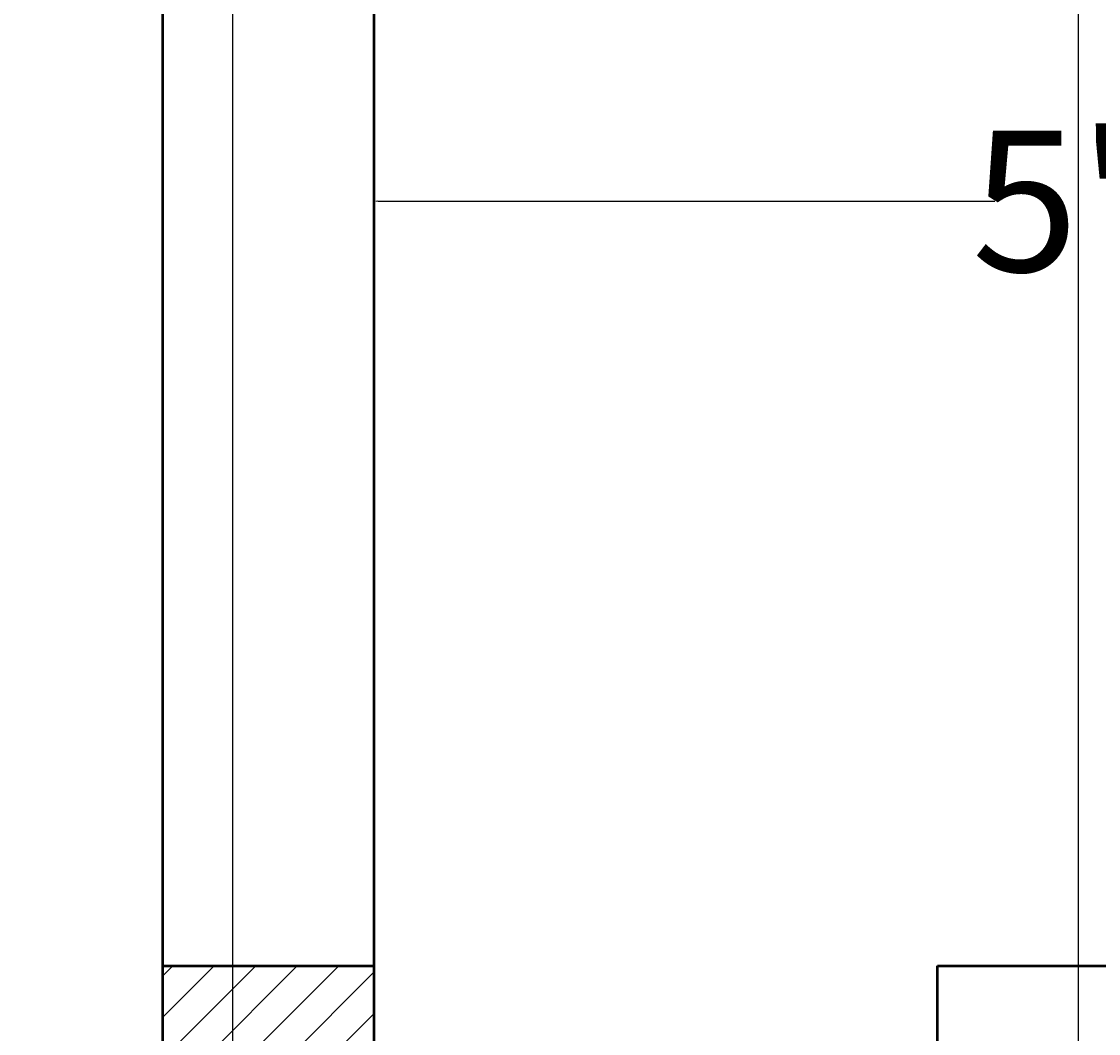
# Model space of a CAD drawing. Units: inches. Extents: x 0 to 281, y -535 to 46.
# Tile 11 of 22: x 150 to 196, y -125 to -82. Entities that reach past the tile are written whole.
import ezdxf

# ---------------------------------------------------------------- set-up
doc = ezdxf.new("R2010")
doc.units = ezdxf.units.IN
doc.header["$MEASUREMENT"] = 0
for name, color, linetype, lineweight in [('A-ANNO-DIMS', 2, 'Continuous', 18), ('A-COLS', 7, 'Continuous', 50), ('A-COLS-PATT', 152, 'Continuous', 13), ('A-WALL', 7, 'Continuous', 50)]:
    doc.layers.add(name, color=color, linetype=linetype, lineweight=lineweight)
doc.styles.get("Standard").update_dxf_attribs({"font": 'arial.ttf'})
doc.dimstyles.get("Standard").update_dxf_attribs({"dimtxt": 0.18, "dimasz": 0.18, "dimexe": 0.18, "dimexo": 0.0625, "dimgap": 0.09, "dimtad": 0, "dimtih": 1, "dimtoh": 1, "dimdec": 0, "dimzin": 0, "dimdsep": 46, "dimlunit": 3, "dimtxsty": 'Standard', "dimcen": 0.09, "dimadec": 0, "dimazin": 0, "dimtfac": 1, "dimtdec": 0, "dimtofl": 0, "dimtmove": 0, "dimatfit": 3, "dimfxl": 1, "dimtolj": 1, "dimtzin": 0, "dimarcsym": 0})

# ---------------------------------------------------------------- blocks, each defined once
blk = doc.blocks.new('*D4')
at = {"layer": 'A-ANNO-DIMS', "color": 0, "lineweight": -2, "transparency": 16777216}
for p, q in [((165.459, -89.775), (165.459, -89.658)), ((165.639, -89.838), (191.894, -89.838)), ((234.279, -89.838), (208.024, -89.838)), ((234.459, -89.775), (234.459, -89.658))]:
    blk.add_line(p, q, dxfattribs=at)
at = {"layer": 'A-ANNO-DIMS', "color": 0, "transparency": 16777216}
for points in [[(165.639, -89.808), (165.639, -89.868), (165.459, -89.838)], [(234.279, -89.808), (234.279, -89.868), (234.459, -89.838)]]:
    blk.add_solid(points, dxfattribs=at)
at = {"layer": 'Defpoints', "color": 0, "transparency": 16777216}
for p in [(165.459, -89.838), (234.459, -89.838), (234.459, -89.838)]:
    blk.add_point(p, dxfattribs=at)
at = {"layer": 'A-ANNO-DIMS', "color": 0, "transparency": 16777216, "insert": (199.959, -89.838), "char_height": 6, "attachment_point": 5}
blk.add_mtext('\\A1;5\'-9"', dxfattribs=at)
blk = doc.blocks.new('*D46')
at = {"layer": 'A-ANNO-DIMS', "color": 0, "lineweight": -2, "transparency": 16777216}
for p, q in [((159.459, -263.348), (159.459, 46.219)), ((159.639, 46.039), (177.13, 46.039)), ((195.279, 46.039), (177.788, 46.039)), ((195.459, -263.348), (195.459, 46.219))]:
    blk.add_line(p, q, dxfattribs=at)
at = {"layer": 'A-ANNO-DIMS', "color": 0, "transparency": 16777216}
for points in [[(159.639, 46.069), (159.639, 46.009), (159.459, 46.039)], [(195.279, 46.069), (195.279, 46.009), (195.459, 46.039)]]:
    blk.add_solid(points, dxfattribs=at)
at = {"layer": 'Defpoints', "color": 0, "transparency": 16777216}
for p in [(195.459, 46.039), (159.459, -263.411), (195.459, -263.411)]:
    blk.add_point(p, dxfattribs=at)
at = {"layer": 'A-ANNO-DIMS', "color": 0, "transparency": 16777216, "insert": (177.459, 46.039), "char_height": 0.18, "attachment_point": 5}
blk.add_mtext('\\A1;3\'-0"', dxfattribs=at)
blk = doc.blocks.new('*D48')
at = {"layer": 'A-ANNO-DIMS', "color": 0, "lineweight": -2, "transparency": 16777216}
for p, q in [((159.459, -392.348), (159.459, 46.219)), ((159.639, 46.039), (177.13, 46.039)), ((195.279, 46.039), (177.788, 46.039)), ((195.459, -392.348), (195.459, 46.219))]:
    blk.add_line(p, q, dxfattribs=at)
at = {"layer": 'A-ANNO-DIMS', "color": 0, "transparency": 16777216}
for points in [[(159.639, 46.069), (159.639, 46.009), (159.459, 46.039)], [(195.279, 46.069), (195.279, 46.009), (195.459, 46.039)]]:
    blk.add_solid(points, dxfattribs=at)
at = {"layer": 'Defpoints', "color": 0, "transparency": 16777216}
for p in [(195.459, 46.039), (159.459, -392.411), (195.459, -392.411)]:
    blk.add_point(p, dxfattribs=at)
at = {"layer": 'A-ANNO-DIMS', "color": 0, "transparency": 16777216, "insert": (177.459, 46.039), "char_height": 0.18, "attachment_point": 5}
blk.add_mtext('\\A1;3\'-0"', dxfattribs=at)

msp = doc.modelspace()

# ---------------------------------------------------------------- hatches: boundary and pattern name
at = {"layer": 'A-COLS-PATT'}
h = msp.add_hatch(dxfattribs=at)
h.set_pattern_fill('ANSI31', color=256, scale=10)
h.paths.add_polyline_path([(165.459, -122.411), (156.459, -122.411), (156.459, -131.411), (165.459, -131.411)])
h.paths.add_polyline_path([(159.459, -263.411), (150.459, -263.411), (150.459, -272.411), (159.459, -272.411)])

# ---------------------------------------------------------------- linework, layer by layer
at = {"layer": 'A-COLS'}
msp.add_line((156.459, -122.411), (165.459, -122.411), dxfattribs=at)
at = {"layer": 'A-WALL'}
for p, q in [((156.459, 18.589), (156.459, -131.411)), ((165.459, 18.589), (165.459, -131.411)), ((189.459, -131.411), (189.459, -122.411)), ((189.459, -122.411), (243.459, -122.411))]:
    msp.add_line(p, q, dxfattribs=at)

# ---------------------------------------------------------------- dimensions: what is measured, and where the dimension line sits
at = {"layer": 'A-ANNO-DIMS'}
for base, p1, p2, override, picture, middle in [((195.459, 46.039), (159.459, -263.411), (195.459, -263.411), {"dimdec": 1, "dimlfac": 1, "dimrnd": 0, "dimzin": 1, "dimdsep": 46, "dimlunit": 4, "dimfrac": 2}, '*D46', (177.459, 46.039)), ((195.459, 46.039), (159.459, -392.411), (195.459, -392.411), {"dimdec": 1, "dimlfac": 1, "dimrnd": 0, "dimzin": 1, "dimdsep": 46, "dimlunit": 4, "dimfrac": 2}, '*D48', (177.459, 46.039)), ((234.459, -89.838), (165.459, -89.838), (234.459, -89.838), {"dimtxt": 6, "dimclrd": 0, "dimclre": 0, "dimclrt": 0}, '*D4', (199.959, -89.838))]:
    dim = msp.add_linear_dim(base=base, p1=p1, p2=p2, dimstyle='Standard', override=override, dxfattribs=at)
    dim.commit()
    dim.dimension.update_dxf_attribs({"geometry": picture, "text_midpoint": middle})

doc.saveas('drawing.dxf')
